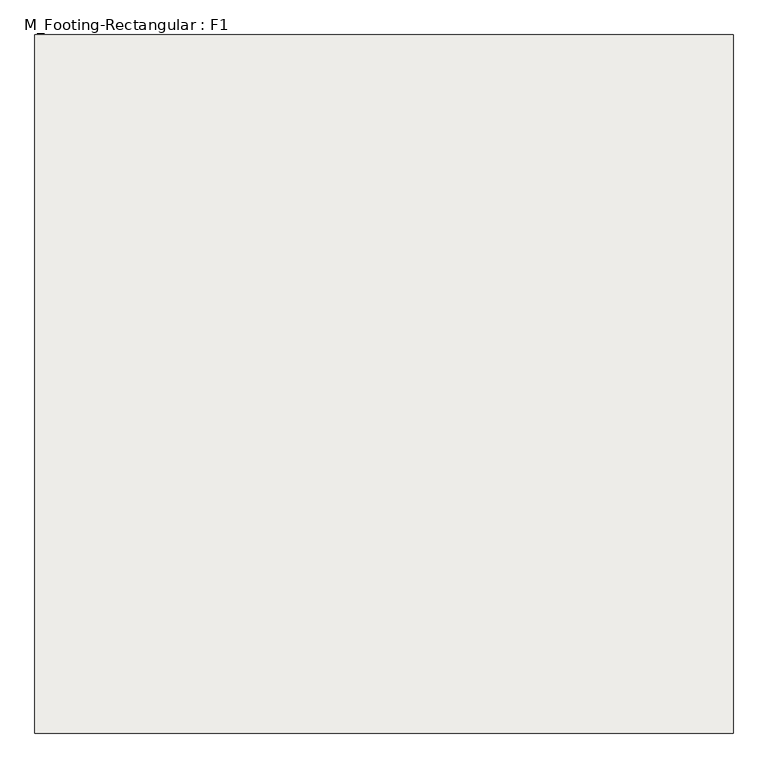
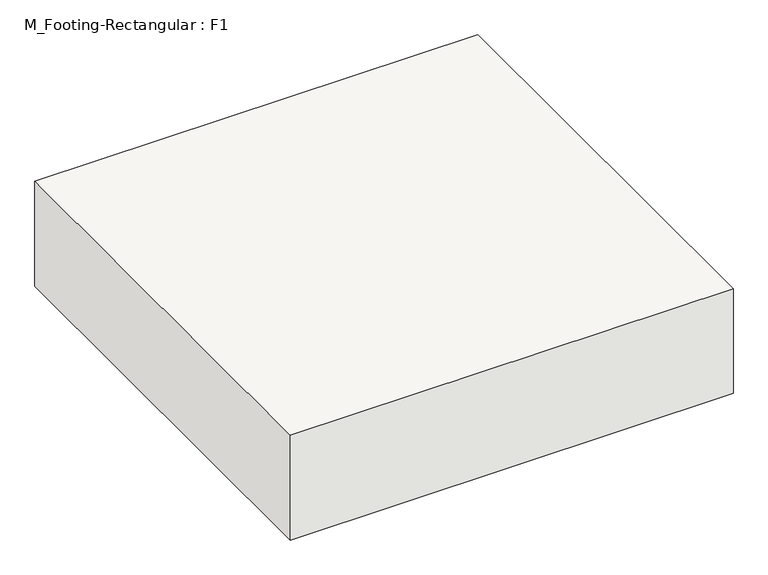
"""IFC4 building model written with IfcOpenShell, lengths in millimetres: slab geometry, M_Footing-Rectangular : F1."""

from ifc_helpers import new_model, si_unit, frame, origin, place, context, project, spatial, polyline, outline, extrude, source, transform, mapped, element, save


def m_footing_rectangular_f1_8f1f0fab(model_context):
    return source(origin(), model_context, "Body", "SweptSolid", [
        extrude(outline(polyline([(1066.8, 1066.8), (1066.8, -1066.8), (-1066.8, -1066.8), (-1066.8, 1066.8), (1066.8, 1066.8)])), frame((0.0, 0.0, -533.4), z_axis=(0.0, 0.0, 1.0), x_axis=(1.0, 0.0, 0.0)), (0.0, 0.0, 1.0), 533.4),
    ])


if __name__ == "__main__":
    model = new_model("IFC4")
    model_context = context("Model", 3, world=origin())
    ifc_project = project(units=[si_unit("LENGTHUNIT", "METRE", prefix="MILLI")], contexts=[model_context])
    site = spatial("IfcSite", under=ifc_project)
    building = spatial("IfcBuilding", under=site)
    placement = place(None, origin())
    m_footing_rectangular_f1_shape = m_footing_rectangular_f1_8f1f0fab(model_context)
    element("IfcSlab", 1, ObjectType="M_Footing-Rectangular : F1", at=placement, inside=building, context=model_context, shape_type="MappedRepresentation", body=[
        mapped(m_footing_rectangular_f1_shape, transform((0.0, 0.0, 0.0), x_axis=(1.0, 0.0, 0.0), y_axis=(0.0, 1.0, 0.0), z_axis=(0.0, 0.0, 1.0))),
    ])
    save(model, "model.ifc")

# Revit data of these elements
# Type "M_Footing-Rectangular : F1"
#   Width = 2133.6 mm
#   Length = 2133.6 mm
#   Foundation Thickness = 533.4 mm
#   Structural Material [instance default] = Concrete, Cast-in-Place gray
#   Assembly Code = ""
# Element 1 (IfcSlab, "M_Footing-Rectangular : F1")
#   Materials on its faces: "Concrete, Cast-in-Place gray"
# Materials
#   "Concrete, Cast-in-Place gray": class "Concrete", colour RGB 192 192 192, transparency 0, Description = "Cast-in-place concrete", Cost = 0
